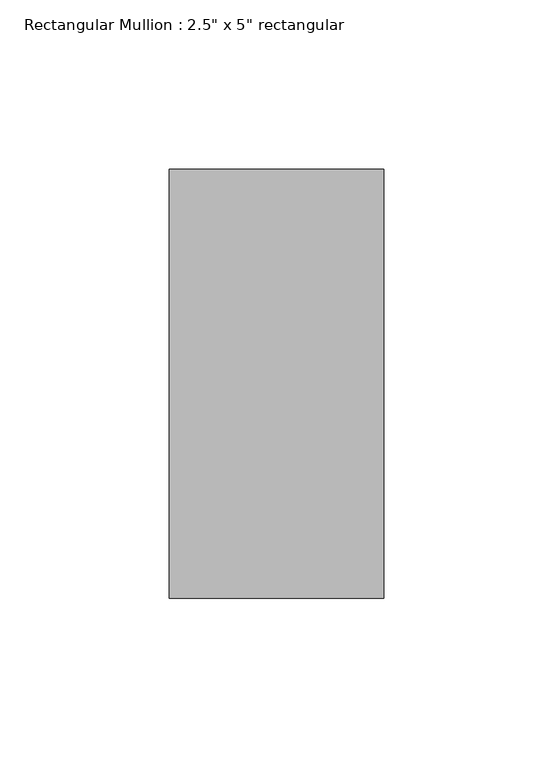
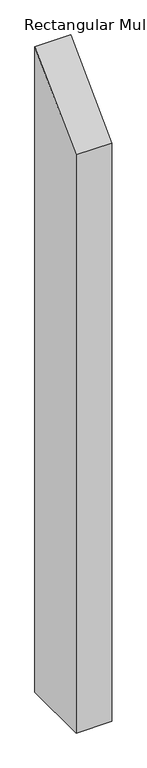
"""IFC4 building model written with IfcOpenShell, lengths in millimetres: member geometry."""

from ifc_helpers import new_model, si_unit, frame, origin, place, context, project, spatial, polyline, outline, extrude, source, transform, mapped, element, save


def member_1d29426d(model_context):
    return source(origin(), model_context, "Body", "SweptSolid", [
        extrude(outline(polyline([(-63.5, -63.5), (63.5, 63.5), (63.5, -1153.7950002), (-63.5, -1153.7950002), (-63.5, -63.5)])), frame((-31.75, 0.0, 0.0), z_axis=(1.0, 0.0, 0.0), x_axis=(0.0, 1.0, 0.0)), (0.0, 0.0, 1.0), 63.5),
    ])


if __name__ == "__main__":
    model = new_model("IFC4")
    model_context = context("Model", 3, world=origin())
    ifc_project = project(units=[si_unit("LENGTHUNIT", "METRE", prefix="MILLI")], contexts=[model_context])
    site = spatial("IfcSite", under=ifc_project)
    building = spatial("IfcBuilding", under=site)
    placement = place(None, origin())
    member_shape = member_1d29426d(model_context)
    element("IfcMember", 1, ObjectType="Rectangular Mullion : 2.5\" x 5\" rectangular", at=placement, inside=building, context=model_context, shape_type="MappedRepresentation", body=[
        mapped(member_shape, transform((0.0, 0.0, 0.0), x_axis=(1.0, 0.0, 0.0), y_axis=(0.0, 1.0, 0.0), z_axis=(0.0, 0.0, 1.0))),
    ])
    save(model, "model.ifc")

# Revit data of these elements
# Type "Rectangular Mullion : 2.5\" x 5\" rectangular"
#   built-in parameter 1007304 = 0.416667 (stored number, unit not read)
#   built-in parameter 1007301 = 0.104167 (stored number, unit not read)
#   built-in parameter 1007300 = 0.104167 (stored number, unit not read)
# Element 1 (IfcMember, "Rectangular Mullion : 2.5\" x 5\" rectangular")
#   Materials on its faces: "Aluminum"
# Materials
#   "Aluminum": class "Metal", colour RGB 247 247 247, transparency 0, Description = "Aluminum 6061", Cost = 0
